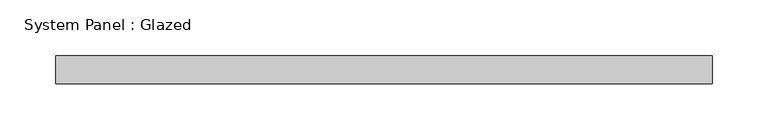
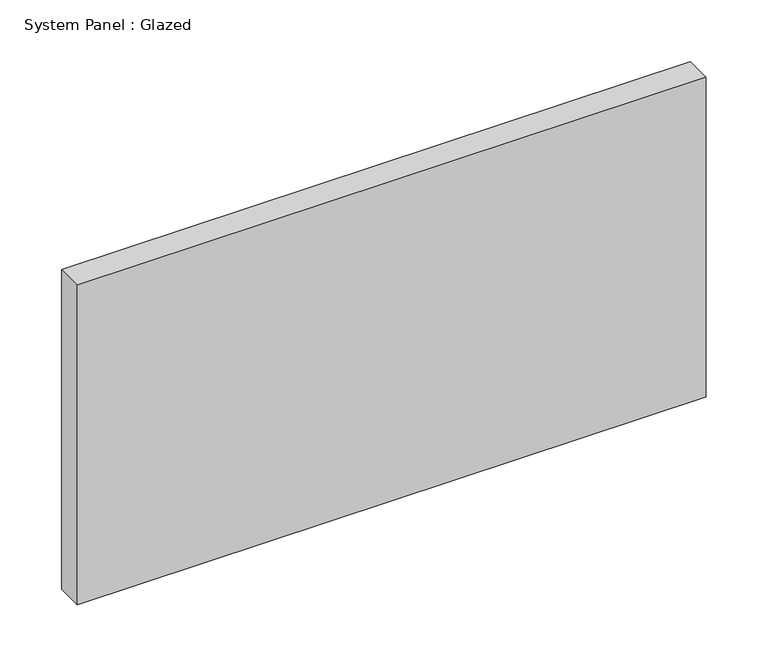
"""IFC4 building model written with IfcOpenShell, lengths in millimetres: plate geometry, System Panel : Glazed."""

from ifc_helpers import new_model, si_unit, origin, origin_with_axes, place, context, project, spatial, polyline, outline, extrude, source, transform, mapped, element, save


def system_panel_glazed_dbf5bbc8(model_context):
    return source(origin(), model_context, "Body", "SweptSolid", [
        extrude(outline(polyline([(295.275, 19.05), (-295.275, 19.05), (-295.275, 44.45), (295.275, 44.45), (295.275, 19.05)])), origin_with_axes(), (0.0, 0.0, 1.0), 317.5),
    ])


if __name__ == "__main__":
    model = new_model("IFC4")
    model_context = context("Model", 3, world=origin())
    ifc_project = project(units=[si_unit("LENGTHUNIT", "METRE", prefix="MILLI")], contexts=[model_context])
    site = spatial("IfcSite", under=ifc_project)
    building = spatial("IfcBuilding", under=site)
    placement = place(None, origin())
    system_panel_glazed_shape = system_panel_glazed_dbf5bbc8(model_context)
    element("IfcPlate", 1, ObjectType="System Panel : Glazed", at=placement, inside=building, context=model_context, shape_type="MappedRepresentation", body=[
        mapped(system_panel_glazed_shape, transform((0.0, 0.0, 0.0), x_axis=(1.0, 0.0, 0.0), y_axis=(0.0, 1.0, 0.0), z_axis=(0.0, 0.0, 1.0))),
    ])
    save(model, "model.ifc")

# Revit data of these elements
# Type "System Panel : Glazed"
#   Construction Type Id = "GSP4R"
#   Analytic Construction = "1/8 in Pilkington single glazing"
#   Visual Light Transmittance = 0.9
#   Solar Heat Gain Coefficient = 0.86
#   Heat Transfer Coefficient (U) = 1.18115 BTU/(h·ft²·°F)
#   Define Thermal Properties by = 1
# Element 1 (IfcPlate, "System Panel : Glazed")
#   Materials on its faces: "Glass"
# Materials
#   "Glass": class "Glass", colour RGB 0 128 192, transparency 0.75, Description = "Soda Lime Glass", Cost = 0
